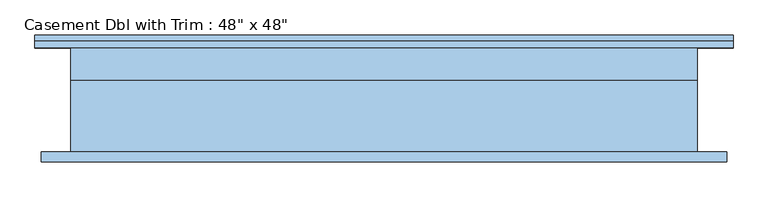
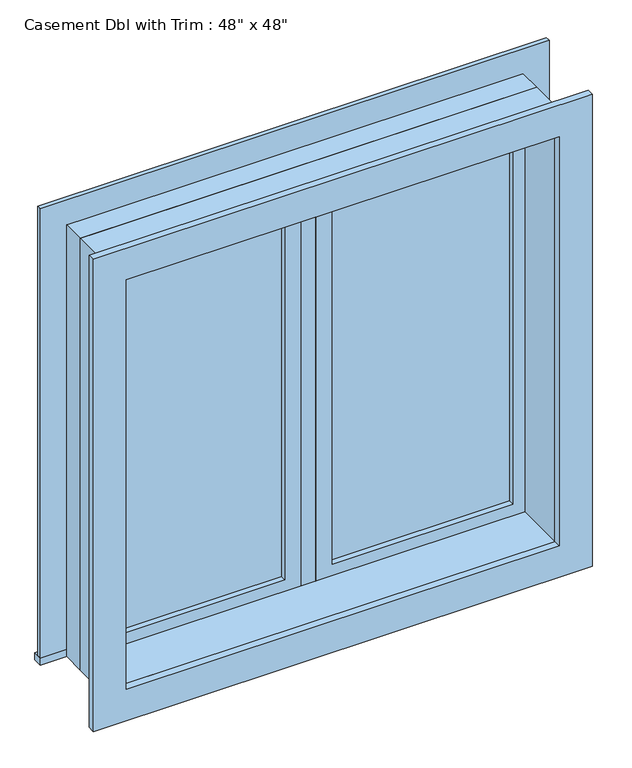
"""IFC4 building model written with IfcOpenShell, lengths in millimetres: window geometry."""

from ifc_helpers import new_model, si_unit, frame, origin, place, context, project, spatial, polyline, outline, extrude, source, transform, mapped, element, save


def window_0862ab64(model_context):
    return source(origin(), model_context, "Body", "SweptSolid", [
        extrude(outline(polyline([(63.5, 85.725), (546.1, 85.725), (546.1, 73.025), (63.5, 73.025), (63.5, 85.725)])), frame((0.0, 0.0, 977.9), z_axis=(0.0, 0.0, 1.0), x_axis=(1.0, 0.0, 0.0)), (0.0, 0.0, 1.0), 1092.2),
        extrude(outline(polyline([(2114.55, 19.05), (933.45, 19.05), (933.45, 590.55), (2114.55, 590.55), (2114.55, 19.05)]), holes=[polyline([(2070.1, 63.5), (2070.1, 546.1), (977.9, 546.1), (977.9, 63.5), (2070.1, 63.5)])]), frame((0.0, 57.15, 0.0), z_axis=(0.0, 1.0, 0.0), x_axis=(0.0, 0.0, 1.0)), (0.0, 0.0, 1.0), 44.45),
        extrude(outline(polyline([(19.05, 57.15), (-19.05, 57.15), (-19.05, 120.65), (19.05, 120.65), (19.05, 57.15)])), frame((0.0, 0.0, 933.45), z_axis=(0.0, 0.0, 1.0), x_axis=(1.0, 0.0, 0.0)), (0.0, 0.0, 1.0), 1181.1),
        extrude(outline(polyline([(-679.45, 146.05), (679.45, 146.05), (679.45, 120.65), (-679.45, 120.65), (-679.45, 146.05)])), frame((0.0, 0.0, 914.4), z_axis=(0.0, 0.0, 1.0), x_axis=(1.0, 0.0, 0.0)), (0.0, 0.0, 1.0), 19.05),
        extrude(outline(polyline([(2114.55, -590.55), (2114.55, 590.55), (933.45, 590.55), (933.45, 679.45), (2203.45, 679.45), (2203.45, -679.45), (933.45, -679.45), (933.45, -590.55), (2114.55, -590.55)])), frame((0.0, 120.65, 0.0), z_axis=(0.0, 1.0, 0.0), x_axis=(0.0, 0.0, 1.0)), (0.0, 0.0, 1.0), 12.7),
        extrude(outline(polyline([(2190.75, 666.75), (2190.75, -666.75), (857.25, -666.75), (857.25, 666.75), (2190.75, 666.75)]), holes=[polyline([(2101.85, 577.85), (946.15, 577.85), (946.15, -577.85), (2101.85, -577.85), (2101.85, 577.85)])]), frame((0.0, -101.6, 0.0), z_axis=(0.0, 1.0, 0.0), x_axis=(0.0, 0.0, 1.0)), (0.0, 0.0, 1.0), 19.05),
        extrude(outline(polyline([(-63.5, 73.025), (-546.1, 73.025), (-546.1, 85.725), (-63.5, 85.725), (-63.5, 73.025)])), frame((0.0, 0.0, 977.9), z_axis=(0.0, 0.0, 1.0), x_axis=(1.0, 0.0, 0.0)), (0.0, 0.0, 1.0), 1092.2),
        extrude(outline(polyline([(2114.55, -590.55), (933.45, -590.55), (933.45, -19.05), (2114.55, -19.05), (2114.55, -590.55)]), holes=[polyline([(2070.1, -546.1), (2070.1, -63.5), (977.9, -63.5), (977.9, -546.1), (2070.1, -546.1)])]), frame((0.0, 57.15, 0.0), z_axis=(0.0, 1.0, 0.0), x_axis=(0.0, 0.0, 1.0)), (0.0, 0.0, 1.0), 44.45),
        extrude(outline(polyline([(2133.6, -609.6), (914.4, -609.6), (914.4, 609.6), (2133.6, 609.6), (2133.6, -609.6)]), holes=[polyline([(2101.85, -577.85), (2101.85, 577.85), (946.15, 577.85), (946.15, -577.85), (2101.85, -577.85)])]), frame((0.0, -82.55, 0.0), z_axis=(0.0, 1.0, 0.0), x_axis=(0.0, 0.0, 1.0)), (0.0, 0.0, 1.0), 139.7),
        extrude(outline(polyline([(2133.6, 609.6), (2133.6, -609.6), (914.4, -609.6), (914.4, 609.6), (2133.6, 609.6)]), holes=[polyline([(2114.55, 590.55), (933.45, 590.55), (933.45, -590.55), (2114.55, -590.55), (2114.55, 590.55)])]), frame((0.0, 57.15, 0.0), z_axis=(0.0, 1.0, 0.0), x_axis=(0.0, 0.0, 1.0)), (0.0, 0.0, 1.0), 63.5),
    ])


if __name__ == "__main__":
    model = new_model("IFC4")
    model_context = context("Model", 3, world=origin())
    ifc_project = project(units=[si_unit("LENGTHUNIT", "METRE", prefix="MILLI")], contexts=[model_context])
    site = spatial("IfcSite", under=ifc_project)
    building = spatial("IfcBuilding", under=site)
    placement = place(None, origin())
    window_shape = window_0862ab64(model_context)
    element("IfcWindow", 1, ObjectType="Casement Dbl with Trim : 48\" x 48\"", at=placement, inside=building, context=model_context, shape_type="MappedRepresentation", body=[
        mapped(window_shape, transform((0.0, 0.0, 0.0), x_axis=(1.0, 0.0, 0.0), y_axis=(0.0, 1.0, 0.0), z_axis=(0.0, 0.0, 1.0))),
    ])
    save(model, "model.ifc")

# Revit data of these elements
# Type "Casement Dbl with Trim : 48\" x 48\""
#   Type Mark = "34"
#   Construction Type Id = "GSP4R"
#   Assembly Code = "B2020100"
#   Analytic Construction = "1/8 in Pilkington single glazing"
#   Visual Light Transmittance = 0.9
#   Solar Heat Gain Coefficient = 0.78
#   Heat Transfer Coefficient (U) = 0.6496 BTU/(h·ft²·°F)
#   Height = 4' - 0"
#   Default Sill Height = 3' - 0"
#   Trim Projection - Ext. = 0' - 0 1/2"
#   Trim Projection - Int. = 0' - 0 3/4"
#   Trim Width - Exterior = 0' - 3 1/2"
#   Trim Width - Interior = 0' - 3 1/2"
#   Width = 4' - 0"
#   Window Inset = 0' - 0 3/4"
#   Define Thermal Properties by = 1
#   Glass Pane Material = Glass
#   Sash Material = Sash
#   Trim Exterior Material = Trim
#   Trim Interior Material = Trim
#   Wall Closure = (empty or 0)
# Element 1 (IfcWindow, "Casement Dbl with Trim : 48\" x 48\"")
#   Materials on its faces: "Sash", "Trim", "Glass"
# Materials
#   "Glass": class "Glass", colour RGB 0 128 192, transparency 0.75, Description = "Soda Lime Glass", Cost = 0
#   "Sash": class "Wood", colour RGB 224 178 126, transparency 0
#   "Trim": class "Wood", colour RGB 224 178 126, transparency 0
